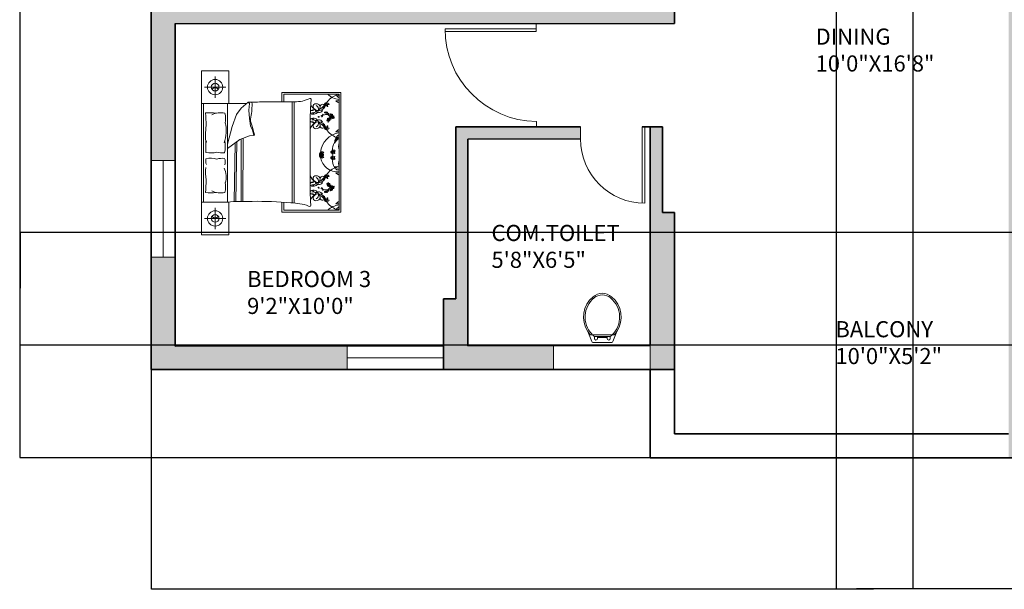
# Model space of a CAD drawing. Units: inches. Extents: x -26 to 13070, y -956 to 6917.
# Tile 1 of 13: x -26 to 341, y -956 to -744. Entities that reach past the tile are written whole.
import ezdxf

# ---------------------------------------------------------------- set-up
doc = ezdxf.new("R2010")
doc.units = ezdxf.units.IN
doc.header["$MEASUREMENT"] = 0
for name, color, linetype, lineweight in [('A-ANNO-DIMS', 2, 'Continuous', 18), ('A-AREA-IDEN', 7, 'Continuous', 18), ('A-DOOR', 3, 'Continuous', 18), ('A-FLOR-FIXT', 9, 'Continuous', 18), ('A-FURN', 8, 'Continuous', 13), ('A-GLAZ', 4, 'Continuous', 18), ('A-WALL', 7, 'Continuous', 35), ('A-WALL-PATT', 252, 'Continuous', 13)]:
    doc.layers.add(name, color=color, linetype=linetype, lineweight=lineweight)
doc.styles.get("Standard").update_dxf_attribs({"font": 'arial.ttf'})
doc.dimstyles.get("Standard").update_dxf_attribs({"dimtxt": 0.18, "dimasz": 0.18, "dimexe": 0.18, "dimexo": 0.0625, "dimgap": 0.09, "dimtad": 0, "dimtih": 1, "dimtoh": 1, "dimdec": 0, "dimzin": 0, "dimdsep": 46, "dimlunit": 3, "dimtxsty": 'Standard', "dimcen": 0.09, "dimadec": 0, "dimazin": 0, "dimtfac": 1, "dimtdec": 0, "dimtofl": 0, "dimtmove": 0, "dimatfit": 3, "dimfxl": 1, "dimtolj": 1, "dimtzin": 0, "dimarcsym": 0})

# ---------------------------------------------------------------- blocks, each defined once
blk = doc.blocks.new('WC-STANDARD')
for p, q in [((2.62, 2.77), (3.39, 2.77)), ((3.39, 2.77), (6.99, 2.77)), ((10.59, 2.77), (6.99, 2.77)), ((10.59, 2.77), (11.36, 2.77))]:
    blk.add_line(p, q)
for points in [[(1.63, 4.03, -0.383919), (3.55, 16.99, -0.163732), (6.99, 18.31, -0.359733)], [(3.02, 3.15, -0.431639), (3.9, 16.57, -0.162618), (6.99, 17.76, -0.470877)], [(12.35, 4.03, 0.383919), (10.43, 16.99, 0.163732), (6.99, 18.31, 0.359733)], [(10.59, 2.77, 0.448546), (10.08, 16.57, 0.162618), (6.99, 17.76, 0.470877)], [(2.62, 2.77, -0.040937), (1.63, 4.03, -0.163732)], [(6.99, 0), (3.49, 0, -0.31031), (3.07, 0.29), (1.63, 4.03, -0.209071)], [(6.99, 0), (10.49, 0, 0.31031), (10.92, 0.29), (12.35, 4.03, 0.209071)], [(11.36, 2.77, 0.040937), (12.35, 4.03, 0.163732)], [(3.39, 2.77, -0.014165), (3.02, 3.15, -0.162618)], [(4.02, 2.22, -0.022712), (3.39, 2.77, -0.162618)], [(6.99, 2.22), (4.02, 2.22, -0.022712)], [(4.02, 2.22), (4.02, 1.45, 1), (5.19, 1.45), (5.19, 1.85)], [(6.99, 2.22), (9.96, 2.22, 0.476108)], [(9.96, 2.22), (9.96, 1.45, -1), (8.79, 1.45), (8.79, 1.85)], [(9.96, 2.22, 0.022712), (10.59, 2.77, 0.162618)]]:
    blk.add_lwpolyline(points, format="xyb")
for points in [[(5.19, 1.85), (5.19, 2.22)], [(8.79, 1.85), (5.19, 1.85)], [(8.79, 1.85), (8.79, 2.22)]]:
    blk.add_lwpolyline(points)
blk = doc.blocks.new('WIN-36')
for p, q in [((0, 36), (0, 0)), ((9, 36), (0, 36)), ((4.5, 36), (4.5, 0)), ((9, 0), (9, 36)), ((0, 0), (9, 0))]:
    blk.add_line(p, q)
blk = doc.blocks.new('*D40')
at = {"layer": 'A-ANNO-DIMS', "color": 0, "lineweight": -2, "transparency": 16777216}
for p, q in [((22.64, -874.6), (22.64, -956.47)), ((547.64, -874.6), (547.64, -956.47)), ((22.82, -956.29), (284.85, -956.29)), ((547.46, -956.29), (285.43, -956.29))]:
    blk.add_line(p, q, dxfattribs=at)
at = {"layer": 'A-ANNO-DIMS', "color": 0, "transparency": 16777216}
for points in [[(22.82, -956.26), (22.82, -956.32), (22.64, -956.29)], [(547.46, -956.26), (547.46, -956.32), (547.64, -956.29)]]:
    blk.add_solid(points, dxfattribs=at)
at = {"layer": 'Defpoints', "color": 0, "transparency": 16777216}
for p in [(22.64, -874.54), (547.64, -874.54), (547.64, -956.29)]:
    blk.add_point(p, dxfattribs=at)
at = {"layer": 'A-ANNO-DIMS', "color": 0, "transparency": 16777216, "insert": (285.14, -956.29), "char_height": 0.18, "attachment_point": 5}
blk.add_mtext('\\A1;525', dxfattribs=at)
blk = doc.blocks.new('*D41')
at = {"layer": 'A-ANNO-DIMS', "color": 0, "lineweight": -2, "transparency": 16777216}
for p, q in [((214.58, 67.46), (-26.29, 67.46)), ((-26.11, 67.28), (-26.11, -419.86)), ((-26.11, -907.36), (-26.11, -420.22)), ((208.58, -907.54), (-26.29, -907.54))]:
    blk.add_line(p, q, dxfattribs=at)
at = {"layer": 'A-ANNO-DIMS', "color": 0, "transparency": 16777216}
for points in [[(-26.14, 67.28), (-26.08, 67.28), (-26.11, 67.46)], [(-26.14, -907.36), (-26.08, -907.36), (-26.11, -907.54)]]:
    blk.add_solid(points, dxfattribs=at)
at = {"layer": 'Defpoints', "color": 0, "transparency": 16777216}
for p in [(-26.11, 67.46), (214.64, 67.46), (208.64, -907.54)]:
    blk.add_point(p, dxfattribs=at)
at = {"layer": 'A-ANNO-DIMS', "color": 0, "transparency": 16777216, "insert": (-26.11, -420.04), "char_height": 0.18, "attachment_point": 5}
blk.add_mtext('\\A1;975', dxfattribs=at)
blk = doc.blocks.new('*D51')
at = {"layer": 'A-ANNO-DIMS', "color": 0, "lineweight": -2, "transparency": 16777216}
for p, q in [((277.92, -535.87), (277.92, -956.47)), ((306.46, -535.87), (306.46, -956.47)), ((278.1, -956.29), (291.8, -956.29)), ((306.28, -956.29), (292.59, -956.29))]:
    blk.add_line(p, q, dxfattribs=at)
at = {"layer": 'A-ANNO-DIMS', "color": 0, "transparency": 16777216}
for points in [[(278.1, -956.26), (278.1, -956.32), (277.92, -956.29)], [(306.28, -956.26), (306.28, -956.32), (306.46, -956.29)]]:
    blk.add_solid(points, dxfattribs=at)
at = {"layer": 'Defpoints', "color": 0, "transparency": 16777216}
for p in [(277.92, -535.8), (306.46, -535.8), (306.46, -956.29)]:
    blk.add_point(p, dxfattribs=at)
at = {"layer": 'A-ANNO-DIMS', "color": 0, "transparency": 16777216, "insert": (292.19, -956.29), "char_height": 0.18, "attachment_point": 5}
blk.add_mtext('\\A1;28.54', dxfattribs=at)
blk = doc.blocks.new('*D59')
at = {"layer": 'A-ANNO-DIMS', "color": 0, "lineweight": -2, "transparency": 16777216}
for p, q in [((538.58, -823.54), (-26.29, -823.54)), ((-26.11, -823.72), (-26.11, -844.36)), ((-26.11, -865.36), (-26.11, -844.72)), ((538.58, -865.54), (-26.29, -865.54))]:
    blk.add_line(p, q, dxfattribs=at)
at = {"layer": 'A-ANNO-DIMS', "color": 0, "transparency": 16777216}
for points in [[(-26.14, -823.72), (-26.08, -823.72), (-26.11, -823.54)], [(-26.14, -865.36), (-26.08, -865.36), (-26.11, -865.54)]]:
    blk.add_solid(points, dxfattribs=at)
at = {"layer": 'Defpoints', "color": 0, "transparency": 16777216}
for p in [(-26.11, -823.54), (538.64, -823.54), (538.64, -865.54)]:
    blk.add_point(p, dxfattribs=at)
at = {"layer": 'A-ANNO-DIMS', "color": 0, "transparency": 16777216, "insert": (-26.11, -844.54), "char_height": 0.18, "attachment_point": 5}
blk.add_mtext('\\A1;42', dxfattribs=at)

msp = doc.modelspace()

# ---------------------------------------------------------------- hatches: boundary and pattern name
at = {"layer": 'A-WALL-PATT'}
h = msp.add_hatch(color=256, dxfattribs=at)
h.dxf.hatch_style = 1
h.paths.add_polyline_path([(223.641, 10.458), (214.641, 10.458), (22.641, 10.458), (22.641, -171.042), (31.641, -171.042), (31.641, -135.042), (205.641, -135.042), (205.641, -241.042), (210.141, -241.042), (210.141, -130.542), (94.641, -130.542), (94.641, -76.542), (85.641, -76.542), (85.641, -126.042), (27.141, -126.042), (27.141, 5.958), (85.641, 5.958), (85.641, -52.542), (94.641, -52.542), (94.641, 1.458), (214.641, 1.458), (214.641, -16.542), (223.641, -16.542), (229.641, -16.542), (229.641, -7.542), (223.641, -7.542)])
h.paths.add_polyline_path([(367.048, 10.458), (346.641, 10.458), (337.641, 10.458), (337.641, -7.542), (331.641, -7.542), (331.641, -16.542), (337.641, -16.542), (342.141, -16.542), (342.141, -128.542), (346.641, -128.542), (346.641, 1.458), (367.048, 1.458)])
h.paths.add_polyline_path([(547.641, 10.458), (403.048, 10.458), (403.048, 1.458), (538.641, 1.458), (538.641, -46.542), (547.641, -46.542)])
h.paths.add_polyline_path([(547.641, -106.542), (538.641, -106.542), (538.641, -154.542), (481.013, -154.542), (481.013, -159.042), (538.641, -159.042), (547.641, -159.042)])
h.paths.add_polyline_path([(457.013, -154.542), (342.141, -154.542), (342.141, -165.042), (346.641, -165.042), (346.641, -159.042), (414.141, -159.042), (414.141, -225.042), (346.641, -225.042), (346.641, -189.042), (342.141, -189.042), (342.141, -234.042), (390.641, -234.042), (390.641, -286.042), (395.141, -286.042), (395.141, -234.042), (456.141, -234.042), (456.141, -312.042), (372.641, -312.042), (372.641, -316.542), (462.641, -316.542), (462.641, -312.042), (460.641, -312.042), (460.641, -234.042), (538.641, -234.042), (547.641, -234.042), (547.641, -195.042), (538.641, -195.042), (538.641, -225.042), (418.641, -225.042), (418.641, -159.042), (457.013, -159.042)])
h.paths.add_polyline_path([(547.641, -270.042), (538.641, -270.042), (538.641, -312.042), (486.641, -312.042), (486.641, -316.542), (538.641, -316.542), (547.641, -316.542)], flags=0)
h.paths.add_polyline_path([(547.641, -456.306), (538.641, -456.306), (538.641, -457.542), (346.641, -457.542), (346.641, -316.542), (346.641, -312.042), (342.141, -312.042), (342.141, -457.542), (145.641, -457.542), (145.641, -466.542), (342.141, -466.542), (342.141, -627.042), (346.641, -627.042), (346.641, -466.542), (538.641, -466.542), (538.641, -514.542), (547.641, -514.542)])
h.paths.add_polyline_path([(466.641, -622.542), (372.641, -622.542), (372.641, -627.042), (388.641, -627.042), (388.641, -721.542), (393.141, -721.542), (393.141, -627.042), (462.141, -627.042), (462.141, -717.042), (466.641, -717.042)])
h.paths.add_polyline_path([(547.641, -574.542), (538.641, -574.542), (538.641, -622.542), (492.641, -622.542), (492.641, -627.042), (538.641, -627.042), (538.641, -654.042), (547.641, -654.042)])
h.paths.add_polyline_path([(547.641, -690.042), (538.641, -690.042), (538.641, -717.042), (466.641, -717.042), (466.641, -721.542), (538.641, -721.542), (538.641, -763.542), (547.641, -763.542)])
h.paths.add_polyline_path([(462.141, -717.042), (419.141, -717.042), (419.141, -721.542), (462.141, -721.542)], flags=0)
h.paths.add_polyline_path([(346.641, -721.542), (352.641, -721.542), (352.641, -717.042), (342.141, -717.042), (342.141, -874.542), (342.141, -907.542), (351.141, -907.542), (351.141, -874.542), (395.949, -874.542), (395.949, -865.542), (351.141, -865.542), (351.141, -841.542), (346.641, -841.542)])
h.paths.add_polyline_path([(547.641, -823.542), (538.641, -823.542), (538.641, -865.542), (431.949, -865.542), (431.949, -874.542), (547.641, -874.542)])
h.paths.add_polyline_path([(172.641, -865.713), (140.641, -865.744), (140.641, -788.744), (182.646, -788.704), (182.641, -784.204), (136.141, -784.249), (136.141, -848.332), (131.641, -848.332), (131.641, -874.542), (172.641, -874.542)])
h.paths.add_polyline_path([(217.641, -816.13), (213.141, -816.13), (213.141, -784.174), (208.641, -784.179), (208.641, -865.679), (208.641, -874.542), (217.641, -874.542)])
h.paths.add_polyline_path([(95.641, -865.788), (31.641, -865.849), (31.641, -832.695), (22.641, -832.695), (22.641, -874.542), (95.641, -874.542)])
h.paths.add_polyline_path([(217.641, -741.17), (31.641, -741.349), (31.641, -708.349), (22.641, -708.349), (22.641, -772.542), (22.641, -796.695), (31.641, -796.695), (31.641, -763.542), (31.641, -745.849), (217.641, -745.67)])
h.paths.add_polyline_path([(31.641, -651.349), (99.65, -651.284), (99.641, -642.284), (31.641, -642.349), (31.641, -639.042), (31.641, -588.349), (125.641, -588.259), (125.641, -651.259), (134.641, -651.25), (134.641, -579.25), (112.641, -579.271), (112.641, -549.042), (112.641, -504.271), (85.633, -504.297), (85.641, -513.297), (103.641, -513.28), (103.641, -549.042), (103.641, -579.28), (31.641, -579.349), (31.641, -549.042), (31.641, -513.349), (49.641, -513.314), (49.633, -504.332), (31.641, -504.349), (22.641, -504.358), (22.641, -684.349), (31.641, -684.349)])
h.paths.add_polyline_path([(31.641, -276.042), (145.641, -276.042), (145.641, -402.042), (145.641, -419.542), (154.641, -419.542), (154.641, -411.042), (154.641, -271.542), (210.141, -271.542), (210.141, -265.042), (205.641, -265.042), (205.641, -267.042), (31.641, -267.042), (31.641, -231.042), (22.641, -231.042), (22.641, -426.852), (31.641, -426.852), (31.641, -411.042), (31.641, -402.042)])

# ---------------------------------------------------------------- linework, layer by layer
at = {"layer": 'A-DOOR'}
for p, q in [((166.16, -747.72), (132.16, -747.72)), ((166.16, -745.72), (166.16, -748.72)), ((166.16, -748.72), (132.16, -748.72)), ((166.197, -784.22), (166.197, -782.22)), ((182.641, -784.179), (182.646, -788.704)), ((205.641, -788.679), (205.641, -784.179)), ((206.641, -788.679), (206.641, -784.179)), ((205.641, -788.679), (205.641, -812.679)), ((206.641, -788.679), (206.641, -812.679))]:
    msp.add_line(p, q, dxfattribs=at)
for centre, radius, start, end in [((166.664, -747.72), 34.503, 180, 269.22602), ((206.641, -788.683), 23.996, 180.04936, 270)]:
    msp.add_arc(centre, radius, start, end, dxfattribs=at)
at = {"layer": 'A-FURN'}
for p, q in [((41.423, -763.315), (41.423, -824.436)), ((46.517, -773.421), (46.517, -765.434)), ((50.51, -769.427), (42.524, -769.427)), ((71.385, -771.383), (71.385, -774.84)), ((93.403, -771.383), (71.385, -771.383)), ((72.093, -774.839), (72.093, -772.091)), ((72.093, -772.091), (92.695, -772.091)), ((92.695, -772.091), (92.695, -815.234)), ((93.403, -815.942), (93.403, -771.383)), ((41.423, -775.539), (58.199, -775.539)), ((42.208, -812.212), (42.208, -775.539)), ((51.082, -775.539), (51.082, -812.212)), ((56.239, -777.221), (54.507, -779.573)), ((58.837, -774.992), (56.239, -777.221)), ((59.332, -775.487), (58.837, -774.992)), ((59.085, -777.963), (59.332, -775.487)), ((75.197, -812.49), (75.197, -774.835)), ((75.96, -812.548), (75.96, -774.835)), ((54.507, -779.573), (52.899, -784.029)), ((59.332, -781.058), (59.085, -777.963)), ((59.703, -783.782), (59.332, -781.058)), ((86.498, -778.114), (85.807, -777.979)), ((52.899, -784.029), (51.082, -790.694)), ((60.446, -785.391), (59.703, -783.782)), ((81.963, -806.284), (81.963, -781.468)), ((86.498, -782.386), (85.807, -782.521)), ((55.744, -788.981), (59.332, -787.62)), ((56.801, -811.996), (56.897, -788.544)), ((59.332, -787.62), (60.941, -787.372)), ((60.941, -787.372), (60.446, -785.391)), ((51.082, -792.331), (55.744, -788.981)), ((53.622, -812.048), (53.927, -790.287)), ((54.249, -812.024), (54.562, -789.831)), ((56.173, -811.993), (56.265, -788.784)), ((86.498, -804.939), (85.807, -804.804)), ((86.498, -809.211), (85.807, -809.346)), ((46.517, -814.331), (46.517, -822.317)), ((71.385, -812.553), (71.385, -815.942)), ((72.093, -815.234), (72.093, -812.54)), ((71.385, -815.942), (93.403, -815.942)), ((92.695, -815.234), (72.093, -815.234)), ((50.51, -818.324), (42.524, -818.324))]:
    msp.add_line(p, q, dxfattribs=at)
for points in [[(51.61, -775.539), (51.61, -763.315), (41.423, -763.315)], [(46.517, -769.427), (45.282, -770.14)], [(46.517, -769.427), (47.752, -770.14)], [(41.423, -812.212), (51.61, -812.212), (51.61, -824.436), (41.423, -824.436)], [(46.517, -818.324), (45.282, -817.611)], [(46.517, -818.324), (47.752, -817.611)]]:
    msp.add_lwpolyline(points, dxfattribs=at)
for points in [[(64.434, -774.864, -0.0012423), (76.031, -774.835, 0.1272016), (81.811, -773.61)], [(42.947, -779.05, -0.0748968), (46.939, -779.124, 0.4728166)], [(47.162, -793.589, -0.1409896), (43.09, -793.712, -0.2352448)], [(47.162, -796.2, 0.1409896), (43.09, -796.077, 0.2352448)], [(42.947, -808.702, 0.0748968), (46.939, -808.627, -0.4728166)], [(74.716, -812.473, -0.0561118), (78.079, -812.916, -0.0953413), (81.318, -813.776)]]:
    msp.add_lwpolyline(points, format="xyb", dxfattribs=at)
for centre, radius in [((46.517, -769.427), 2.852), ((46.517, -769.427), 1.426), ((90.353, -780.627), 0.156), ((88.713, -781.645), 0.156), ((88.713, -805.68), 0.156), ((90.353, -806.698), 0.156), ((46.517, -818.324), 2.852), ((46.517, -818.324), 1.426)]:
    msp.add_circle(centre, radius, dxfattribs=at)
for centre, radius, start, end in [((81.772, -774.172), 0.564, 332.65876, 86.02002), ((94.559, -779.804), 7.982, 111.40921, 145.61345), ((93.77, -766.149), 7.982, 228.1144, 262.25504), ((94.839, -770.153), 3.889, 209.88843, 236.53828), ((95.564, -768.754), 4.847, 223.51858, 233.69643), ((60.357, -718.951), 56.062, 268.44695, 274.17059), ((37.193, -776.038), 23.068, 348.6608, 2.54812), ((145.587, -780.738), 63.628, 174.31131, 180.65675), ((86.268, -773.934), 4.626, 206.70034, 236.33288), ((84.046, -776.629), 1.032, 88.94622, 185.51443), ((84.81, -776.312), 1.838, 193.079, 274.70666), ((84.194, -777.052), 1.461, 7.11425, 95.05515), ((83.64, -777.626), 1.418, 338.57785, 68.41813), ((83.869, -776.798), 1.775, 305.95986, 357.6409), ((84.761, -774.87), 3.28, 273.4924, 303.71172), ((84.528, -774.897), 2.886, 288.2955, 328.73863), ((86.548, -776.716), 0.917, 19.13116, 189.73602), ((86.271, -776.496), 1.145, 285.6955, 4.03098), ((87.794, -777.73), 1.22, 128.41745, 173.8338), ((87.541, -776.527), 0.562, 126.73195, 206.02445), ((87.816, -775.939), 0.662, 76.27204, 177.04841), ((86.809, -774.586), 1.363, 284.70312, 328.61733), ((88.71, -776.32), 1.262, 125.76571, 194.53465), ((82.522, -774.086), 5.584, 332.81761, 347.48274), ((88.161, -776.161), 0.885, 20.96132, 102.28847), ((88.639, -775.276), 0.667, 181.71311, 301.53669), ((86.453, -776.625), 2.019, 2.0648, 41.15983), ((87.669, -775.874), 0.653, 316.22381, 62.3173), ((88.078, -776.266), 0.0863, 20.28165, 316.22381), ((88.371, -776.556), 0.0991, 168.5166, 2.0648), ((88.321, -776.545), 0.0482, 52.05911, 168.5166), ((93.939, -772.331), 3.245, 221.04544, 247.44526), ((92.195, -763.442), 11.043, 266.34809, 272.59189), ((-538.724, -812.74), 582.646, 2.850225, 3.314791), ((48.542, -786.837), 7.878, 78.24166, 114.8684), ((42.231, -781.23), 8.191, 348.96311, 14.89607), ((64.689, -781.552), 4.975, 168.6608, 203.73842), ((82.64, -781.733), 0.736, 134.45169, 156.77099), ((82.64, -778.767), 0.736, 206.44199, 225.54831), ((82.64, -778.767), 0.736, 127.67503, 149.9707), ((82.416, -775.631), 2.532, 260.84458, 301.17822), ((83.074, -777.592), 1.948, 240.8249, 340.71782), ((82.494, -778.456), 0.915, 246.16459, 318.43469), ((83.074, -782.908), 1.948, 19.28218, 119.1751), ((82.494, -782.044), 0.915, 41.56531, 113.83541), ((83.515, -780.134), 2.357, 85.26963, 124.21495), ((83.426, -777.298), 1.757, 240.08513, 262.56401), ((84.115, -779.894), 1.253, 74.85287, 138.43469), ((85.181, -777.356), 1.52, 196.8663, 330.09146), ((84.542, -778.319), 0.379, 254.85287, 12.69594), ((83.515, -780.134), 2.357, 53.65552, 57.29887), ((85.045, -780.412), 0.192, 169.58644, 349.56155), ((85.117, -780.425), 0.118, 349.56155, 167.29493), ((88.194, -784.662), 5.062, 110.10592, 116.9968), ((86.496, -780.489), 0.321, 129.50559, 182.64212), ((85.575, -779.747), 0.966, 308.43876, 328.83597), ((85.406, -778.962), 1.724, 296.50636, 305.31021), ((85.392, -779.848), 0.982, 336.39009, 344.48709), ((86.462, -780.099), 0.125, 83.94573, 185.62162), ((85.963, -779.982), 0.512, 328.83597, 0.81412), ((86.228, -780.132), 0.293, 306.52319, 32.46683), ((86.578, -779.905), 0.125, 112.55835, 214.23425), ((86.497, -779.682), 0.293, 265.71315, 351.65678), ((86.24, -779.52), 0.512, 297.36586, 329.34401), ((85.852, -779.08), 0.982, 313.69288, 321.78988), ((86.938, -779.75), 0.321, 115.53786, 168.67439), ((85.849, -779.289), 0.966, 329.34401, 349.74122), ((88.194, -784.662), 5.062, 86.17232, 106.41582), ((85.077, -779.511), 1.724, 352.86976, 1.67361), ((87.361, -778.889), 0.12, 125.0752, 284.76444), ((87.547, -778.843), 0.26, 127.3642, 168.43627), ((87.343, -778.634), 0.374, 277.49685, 341.27373), ((87.64, -778.809), 0.149, 88.13253, 178.89195), ((87.939, -778.967), 0.322, 136.34618, 189.6513), ((87.754, -778.998), 0.134, 189.6513, 312.32085), ((87.788, -778.628), 0.156, 183.27684, 356.72316), ((88.274, -778.906), 0.51, 164.28291, 186.91484), ((87.673, -778.909), 0.255, 312.32085, 40.21108), ((88.213, -778.622), 0.362, 201.63824, 274.94696), ((87.734, -779.117), 0.473, 42.38963, 66.57243), ((92.501, -775.377), 5.803, 217.9541, 226.84587), ((88.076, -778.84), 0.257, 10.95974, 52.23791), ((88.233, -778.864), 0.119, 274.94696, 37.52629), ((88.481, -780.454), 0.71, 253.63009, 325.46314), ((88.681, -781.439), 0.502, 82.07481, 142.68955), ((88.624, -780.749), 0.516, 228.34199, 274.98936), ((88.439, -781.45), 0.153, 138.29465, 276.24744), ((88.496, -781.473), 0.212, 358.57189, 143.89544), ((88.62, -781.306), 0.214, 208.84925, 269.93549), ((88.635, -779.541), 0.125, 112.55835, 214.23425), ((88.554, -779.318), 0.293, 265.71315, 351.65678), ((88.296, -779.156), 0.512, 297.36586, 329.34401), ((88.321, -782.14), 2.538, 60.79592, 85.24398), ((82.918, -785.794), 8.351, 37.82556, 47.75876), ((87.909, -778.716), 0.982, 313.69288, 321.78988), ((88.64, -780.832), 0.431, 273.87739, 357.15012), ((88.995, -779.386), 0.321, 115.53786, 168.67439), ((89.183, -781.604), 0.491, 121.9501, 165.24419), ((87.906, -778.925), 0.966, 329.34401, 349.74122), ((88.807, -780.528), 0.418, 262.07481, 308.23927), ((88.844, -781.415), 0.103, 262.86802, 7.09399), ((87.134, -779.147), 1.724, 352.86976, 1.67361), ((88.831, -781.328), 0.307, 278.56141, 22.59143), ((91.692, -782.401), 3.044, 156.15226, 156.94993), ((89.005, -781.318), 0.154, 44.37319, 121.9501), ((89.481, -780.956), 0.431, 181.4625, 249.4747), ((89.407, -780.616), 0.418, 215.11283, 261.27729), ((89.741, -780.638), 0.71, 197.88895, 269.722), ((91.692, -782.401), 3.044, 130.18202, 149.45598), ((89.52, -780.88), 0.516, 248.36273, 295.0101), ((89.268, -781.525), 0.502, 20.66254, 81.27729), ((89.558, -779.494), 0.174, 33.09787, 123.13641), ((85.729, -781.945), 4.547, 31.11559, 34.8118), ((89.306, -779.793), 0.471, 2.31716, 70.52013), ((90.016, -780.667), 0.502, 139.38119, 199.99593), ((89.08, -780.303), 0.71, 310.93647, 22.76952), ((89.405, -780.342), 0.516, 285.64837, 332.29574), ((89.694, -779.908), 0.136, 135.73542, 318.12966), ((89.468, -779.688), 0.18, 315.73542, 31.11559), ((89.318, -780.069), 0.418, 319.38119, 5.54564), ((89.796, -779.908), 0.136, 68.24522, 250.63946), ((89.484, -779.74), 0.405, 352.60083, 57.18452), ((90.931, -782.46), 2.711, 111.70871, 116.21806), ((88.321, -782.14), 2.538, 47.50829, 55.99666), ((89.871, -779.649), 0.405, 252.8042, 349.69432), ((89.484, -780.374), 0.431, 331.18377, 51.67918), ((89.927, -780.889), 0.12, 125.0752, 284.76444), ((89.913, -779.615), 0.18, 248.24522, 323.62539), ((90.112, -780.842), 0.26, 93.63497, 168.43627), ((90.079, -780.432), 0.153, 138.29465, 276.24744), ((89.755, -779.504), 0.471, 291.70871, 3.02993), ((89.909, -780.634), 0.374, 277.49685, 341.27373), ((90.137, -780.455), 0.212, 358.57189, 143.89544), ((90.206, -780.808), 0.149, 88.13253, 178.89195), ((86.397, -777.024), 4.547, 323.62539, 327.3216), ((90.26, -780.288), 0.214, 208.84925, 269.93549), ((90.078, -780.339), 0.245, 274.21229, 318.15875), ((90.505, -780.966), 0.322, 136.34618, 189.6513), ((90.32, -780.998), 0.134, 189.6513, 312.32085), ((90.126, -779.623), 0.174, 325.60767, 55.6462), ((90.84, -780.905), 0.51, 164.28291, 186.91484), ((90.824, -780.586), 0.491, 121.9501, 165.24419), ((90.239, -780.909), 0.255, 312.32085, 40.21108), ((90.778, -780.622), 0.362, 201.63824, 274.94696), ((90.485, -780.397), 0.103, 262.86802, 7.09399), ((90.299, -781.117), 0.473, 42.38963, 66.57243), ((90.472, -780.31), 0.307, 278.56141, 22.59143), ((90.642, -780.839), 0.257, 10.95974, 118.78041), ((90.646, -780.3), 0.154, 44.37319, 121.9501), ((90.799, -780.863), 0.119, 274.94696, 37.52629), ((65.064, -787.425), 22.167, 170.50302, 187.78042), ((36.409, -785.542), 14.207, 340.73848, 11.96026), ((37.844, -791.616), 23.703, 10.66171, 19.88058), ((82.64, -781.733), 0.736, 203.28564, 232.32497), ((82.416, -784.869), 2.532, 58.82178, 100.28665), ((86.268, -786.566), 4.626, 123.66712, 158.50587), ((83.515, -780.366), 2.357, 235.78505, 274.73037), ((83.426, -783.202), 1.757, 97.43599, 119.91487), ((84.046, -783.871), 1.032, 174.48557, 271.05378), ((84.81, -784.188), 1.838, 85.29334, 166.921), ((84.115, -780.606), 1.253, 221.56531, 285.14713), ((85.181, -783.143), 1.52, 29.90854, 163.1337), ((84.194, -783.448), 1.461, 264.94485, 352.88575), ((83.64, -782.874), 1.418, 291.58187, 21.42215), ((84.542, -782.181), 0.379, 347.30406, 105.14713), ((83.515, -780.366), 2.357, 302.70113, 306.34448), ((83.869, -783.702), 1.775, 2.3591, 54.04014), ((84.761, -785.629), 3.28, 56.28828, 86.5076), ((84.528, -785.602), 2.886, 31.26137, 71.7045), ((86.548, -783.784), 0.917, 170.26398, 340.86884), ((87.794, -782.77), 1.22, 186.1662, 231.58255), ((86.271, -784.004), 1.145, 355.96902, 74.3045), ((87.541, -783.973), 0.562, 153.97555, 233.26805), ((87.816, -784.561), 0.662, 182.95159, 283.72796), ((86.809, -785.913), 1.363, 31.38267, 75.29688), ((88.71, -784.18), 1.262, 165.46535, 234.23429), ((82.522, -786.414), 5.584, 12.51726, 27.18239), ((86.453, -783.875), 2.019, 318.84017, 357.9352), ((87.669, -784.625), 0.653, 297.6827, 43.77619), ((88.639, -785.223), 0.667, 58.46331, 178.28689), ((88.161, -784.339), 0.885, 257.71153, 339.03868), ((88.045, -784.243), 0.052, 43.77292, 339.73329), ((88.286, -781.907), 0.12, 125.0752, 284.76444), ((88.472, -781.86), 0.26, 93.63497, 168.43627), ((88.371, -783.944), 0.0991, 357.9352, 191.4834), ((88.321, -783.954), 0.0482, 191.4834, 307.94089), ((88.268, -781.652), 0.374, 277.49685, 341.27373), ((88.565, -781.827), 0.149, 88.13253, 178.89195), ((88.437, -781.357), 0.245, 274.21229, 318.15875), ((88.864, -781.985), 0.322, 136.34618, 189.6513), ((88.679, -782.016), 0.134, 189.6513, 312.32085), ((91.692, -782.401), 3.044, 175.24147, 182.89291), ((89.199, -781.923), 0.51, 164.28291, 186.91484), ((88.598, -781.927), 0.255, 312.32085, 40.21108), ((89.138, -781.64), 0.362, 201.63824, 274.94696), ((88.659, -782.135), 0.473, 42.38963, 66.57243), ((89.001, -781.857), 0.257, 10.95974, 118.78041), ((89.158, -781.881), 0.119, 274.94696, 37.52629), ((60.991, -787.233), 0.147, 250.24637, 1.13765), ((93.77, -794.351), 7.982, 97.74496, 175.53767), ((94.559, -780.696), 7.982, 214.38655, 248.59079), ((94.839, -790.347), 3.889, 123.46172, 178.72803), ((95.564, -791.746), 4.847, 126.30357, 162.14962), ((96.927, -794.293), 7.209, 125.94696, 145.98766), ((93.939, -788.169), 3.245, 112.55474, 138.95456), ((92.195, -797.058), 11.043, 87.40811, 93.65191), ((53.862, -792.107), 10.891, 166.04004, 188.47507), ((39.511, -791.294), 10.778, 346.37624, 10.13831), ((98.045, -793.74), 7.982, 152.5854, 175.53767), ((96.891, -791.508), 4.389, 162.9798, 196.45689), ((45.995, -796.916), 3.024, 163.89744, 206.65626), ((49.205, -786.384), 7.489, 254.17072, 275.98711), ((49.205, -803.405), 7.489, 84.01289, 105.82928), ((47.049, -797.325), 3.24, 341.45927, 24.98174), ((85.997, -794.365), 0.662, 106.19625, 206.97263), ((85.997, -794.997), 0.662, 153.02737, 253.80375), ((84.45, -793.695), 1.363, 314.62734, 358.54154), ((84.45, -795.667), 1.363, 1.45846, 45.37266), ((86.963, -794.249), 1.262, 155.68992, 224.45887), ((86.963, -795.113), 1.262, 135.54113, 204.31008), ((86.407, -794.386), 0.885, 50.88554, 132.21268), ((86.38, -793.38), 0.667, 211.63732, 331.4609), ((85.838, -794.382), 0.653, 346.14802, 92.24151), ((80.485, -795.4), 5.584, 2.74183, 17.40696), ((85.158, -795.64), 2.019, 31.98902, 71.08405), ((80.485, -793.962), 5.584, 342.59304, 357.25817), ((85.158, -793.723), 2.019, 288.91595, 328.01098), ((85.838, -794.98), 0.653, 267.75849, 13.85198), ((86.38, -795.982), 0.667, 28.5391, 148.36268), ((86.407, -794.977), 0.885, 227.78732, 309.11446), ((91.927, -794.754), 6.177, 188.18034, 277.13645), ((86.388, -794.518), 0.0863, 50.07546, 346.14802), ((86.355, -794.836), 0.052, 13.97912, 309.80908), ((86.738, -794.639), 0.0482, 81.98332, 198.44082), ((86.738, -794.724), 0.0482, 161.55918, 278.01668), ((86.786, -794.623), 0.0991, 198.44082, 31.98902), ((86.786, -794.74), 0.0991, 328.01098, 161.55918), ((90.272, -793.754), 0.662, 106.19625, 206.97263), ((90.272, -795.608), 0.662, 153.02737, 253.80375), ((88.725, -793.084), 1.363, 314.62734, 358.54154), ((88.725, -796.278), 1.363, 1.45846, 45.37266), ((91.238, -793.638), 1.262, 155.68992, 224.45887), ((91.238, -795.724), 1.262, 135.54113, 204.31008), ((90.683, -793.774), 0.885, 50.88554, 132.21268), ((90.655, -792.769), 0.667, 211.63732, 331.4609), ((90.113, -793.771), 0.653, 346.14802, 92.24151), ((89.433, -795.028), 2.019, 31.98902, 71.08405), ((84.76, -794.789), 5.584, 2.74183, 17.40696), ((84.76, -794.573), 5.584, 342.59304, 357.25817), ((89.433, -794.334), 2.019, 288.91595, 328.01098), ((90.113, -795.591), 0.653, 267.75849, 13.85198), ((90.655, -796.593), 0.667, 28.5391, 148.36268), ((90.663, -793.907), 0.0863, 50.07546, 346.14802), ((90.63, -795.447), 0.052, 13.97912, 309.80908), ((91.013, -794.028), 0.0482, 81.98332, 198.44082), ((91.013, -795.335), 0.0482, 161.55918, 278.01668), ((91.061, -794.012), 0.0991, 198.44082, 31.98902), ((91.061, -795.351), 0.0991, 328.01098, 161.55918), ((99.153, -793.246), 6.49, 174.36426, 175.62128), ((103.599, -796.665), 11.598, 160.09716, 160.27829), ((53.642, -801.447), 10.745, 168.8159, 193.65729), ((42.835, -802.986), 7.78, 343.82536, 26.12389), ((94.559, -806.629), 7.982, 111.40921, 145.61345), ((90.683, -795.588), 0.885, 227.78732, 309.11446), ((98.045, -795.623), 7.982, 184.46233, 207.4146), ((91.363, -795.552), 3.573, 263.38046, 291.88297), ((92.357, -798.83), 1.433, 190.92615, 283.61018), ((92.161, -797.754), 1.812, 228.09513, 287.13912), ((96.891, -797.855), 4.389, 163.54311, 197.0202), ((99.153, -796.116), 6.49, 184.37872, 185.63574), ((103.599, -792.698), 11.598, 199.72171, 199.90284), ((86.268, -800.759), 4.626, 201.49413, 236.33288), ((84.046, -803.454), 1.032, 88.94622, 185.51443), ((84.194, -803.877), 1.461, 7.11425, 95.05515), ((83.64, -804.451), 1.418, 338.57785, 68.41813), ((84.528, -801.723), 2.886, 288.2955, 328.73863), ((86.548, -803.541), 0.917, 19.13116, 189.73602), ((86.271, -803.321), 1.145, 285.6955, 4.03098), ((87.541, -803.353), 0.562, 126.73195, 206.02445), ((87.816, -802.764), 0.662, 76.27204, 177.04841), ((86.809, -801.412), 1.363, 284.70312, 328.61733), ((88.71, -803.145), 1.262, 125.76571, 194.53465), ((82.522, -800.911), 5.584, 332.81761, 347.48274), ((88.161, -802.986), 0.885, 20.96132, 102.28847), ((87.669, -802.7), 0.653, 316.22381, 62.3173), ((86.453, -803.45), 2.019, 2.0648, 41.15983), ((88.639, -802.102), 0.667, 181.71311, 301.53669), ((88.078, -803.092), 0.0863, 20.28165, 316.22381), ((88.371, -803.381), 0.0991, 168.5166, 2.0648), ((88.321, -803.371), 0.0482, 52.05911, 168.5166), ((92.195, -790.267), 11.043, 266.34809, 272.59189), ((93.939, -799.156), 3.245, 221.04544, 247.44526), ((-538.724, -775.012), 582.646, 356.685209, 357.149775), ((42.231, -806.521), 8.191, 345.10393, 11.03689), ((141.409, -808.156), 59.476, 178.19649, 184.75976), ((82.416, -802.456), 2.532, 259.71335, 301.17822), ((82.64, -805.593), 0.736, 127.67503, 156.71436), ((82.64, -805.593), 0.736, 203.28564, 225.54831), ((83.074, -804.417), 1.948, 240.8249, 340.71782), ((82.494, -805.281), 0.915, 246.16459, 318.43469), ((83.515, -806.959), 2.357, 85.26963, 124.21495), ((83.426, -804.123), 1.757, 240.08513, 262.56401), ((84.81, -803.137), 1.838, 193.079, 274.70666), ((84.115, -806.72), 1.253, 74.85287, 138.43469), ((85.181, -804.182), 1.52, 196.8663, 330.09146), ((84.542, -805.144), 0.379, 254.85287, 12.69594), ((83.515, -806.959), 2.357, 53.65552, 57.29887), ((85.045, -806.913), 0.192, 10.43845, 190.41356), ((83.869, -803.623), 1.775, 305.95986, 357.6409), ((84.761, -801.696), 3.28, 273.4924, 303.71172), ((85.117, -806.9), 0.118, 192.70507, 10.43845), ((85.575, -807.578), 0.966, 31.16403, 51.56124), ((86.496, -806.836), 0.321, 177.35788, 230.49441), ((85.406, -808.363), 1.724, 54.68979, 63.49364), ((85.392, -807.477), 0.982, 15.51291, 23.60991), ((85.963, -807.343), 0.512, 359.18588, 31.16403), ((86.228, -807.193), 0.293, 327.53317, 53.47681), ((87.794, -804.555), 1.22, 128.41745, 173.8338), ((88.286, -805.418), 0.12, 75.23556, 234.9248), ((88.472, -805.465), 0.26, 191.56373, 266.36503), ((88.624, -806.576), 0.516, 85.01064, 131.65801), ((88.481, -806.871), 0.71, 34.53686, 106.36991), ((88.681, -805.886), 0.502, 217.31045, 277.92519), ((88.439, -805.875), 0.153, 83.75256, 221.70535), ((88.268, -805.673), 0.374, 18.72627, 82.50315), ((88.496, -805.852), 0.212, 216.10456, 1.42811), ((88.565, -805.498), 0.149, 181.10805, 271.86747), ((88.62, -806.019), 0.214, 90.06451, 151.15075), ((88.437, -805.968), 0.245, 41.84125, 85.78771), ((82.918, -801.532), 8.351, 312.24124, 322.17444), ((88.864, -805.341), 0.322, 170.3487, 223.65382), ((88.679, -805.309), 0.134, 47.67915, 170.3487), ((91.692, -804.924), 3.044, 177.10709, 184.75853), ((88.64, -806.493), 0.431, 2.84988, 86.12261), ((89.199, -805.402), 0.51, 173.08516, 195.71709), ((89.183, -805.721), 0.491, 194.75581, 238.0499), ((88.807, -806.797), 0.418, 51.76073, 97.92519), ((88.598, -805.398), 0.255, 319.78892, 47.67915), ((89.138, -805.685), 0.362, 85.05304, 158.36176), ((88.844, -805.91), 0.103, 352.90601, 97.13198), ((88.659, -805.19), 0.473, 293.42757, 317.61037), ((89.001, -805.468), 0.257, 241.21959, 349.04026), ((88.831, -805.997), 0.307, 337.40857, 81.43859), ((91.692, -804.924), 3.044, 203.05007, 203.84774), ((89.005, -806.007), 0.154, 238.0499, 315.62681), ((89.481, -806.37), 0.431, 110.5253, 178.5375), ((89.741, -806.687), 0.71, 90.278, 162.11105), ((89.407, -806.709), 0.418, 98.72271, 144.88717), ((91.692, -804.924), 3.044, 210.54402, 229.81798), ((89.158, -805.444), 0.119, 322.47371, 85.05304), ((89.52, -806.445), 0.516, 64.9899, 111.63727), ((89.268, -805.801), 0.502, 278.72271, 339.33746), ((90.016, -806.658), 0.502, 160.00407, 220.61881), ((89.08, -807.022), 0.71, 337.23048, 49.06353), ((89.405, -806.983), 0.516, 27.70426, 74.35163), ((89.318, -807.256), 0.418, 354.45436, 40.61881), ((88.321, -805.185), 2.538, 304.00334, 312.49171), ((89.484, -806.951), 0.431, 308.32082, 28.81623), ((89.927, -806.436), 0.12, 75.23556, 234.9248), ((90.112, -806.483), 0.26, 191.56373, 266.36503), ((90.079, -806.893), 0.153, 83.75256, 221.70535), ((89.909, -806.691), 0.374, 18.72627, 82.50315), ((90.137, -806.87), 0.212, 216.10456, 1.42811), ((90.206, -806.517), 0.149, 181.10805, 271.86747), ((90.26, -807.037), 0.214, 90.06451, 151.15075), ((90.078, -806.986), 0.245, 41.84125, 85.78771), ((90.505, -806.359), 0.322, 170.3487, 223.65382), ((90.32, -806.327), 0.134, 47.67915, 170.3487), ((90.84, -806.42), 0.51, 173.08516, 195.71709), ((90.824, -806.74), 0.491, 194.75581, 238.0499), ((90.239, -806.416), 0.255, 319.78892, 47.67915), ((90.778, -806.703), 0.362, 85.05304, 158.36176), ((90.485, -806.929), 0.103, 352.90601, 97.13198), ((90.299, -806.209), 0.473, 293.42757, 317.61037), ((90.642, -806.486), 0.257, 241.21959, 349.04026), ((90.472, -807.015), 0.307, 337.40857, 81.43859), ((90.799, -806.462), 0.119, 322.47371, 85.05304), ((48.542, -800.915), 7.878, 245.1316, 281.75834), ((82.64, -808.558), 0.736, 134.45169, 163.36566), ((82.64, -808.558), 0.736, 197.41857, 232.32497), ((82.416, -811.694), 2.532, 58.82178, 100.75101), ((86.268, -813.391), 4.626, 123.66712, 156.35467), ((83.074, -809.733), 1.948, 19.28218, 119.1751), ((82.494, -808.869), 0.915, 41.56531, 113.83541), ((83.515, -807.191), 2.357, 235.78505, 274.73037), ((83.426, -810.027), 1.757, 97.43599, 119.91487), ((84.046, -810.696), 1.032, 174.48557, 271.05378), ((84.81, -811.013), 1.838, 85.29334, 166.921), ((84.115, -807.431), 1.253, 221.56531, 285.14713), ((85.181, -809.969), 1.52, 29.90854, 163.1337), ((84.194, -810.273), 1.461, 264.94485, 352.88575), ((83.64, -809.699), 1.418, 291.58187, 21.42215), ((84.542, -809.007), 0.379, 347.30406, 105.14713), ((83.515, -807.191), 2.357, 302.70113, 306.34448), ((83.869, -810.527), 1.775, 2.3591, 54.04014), ((84.761, -812.455), 3.28, 56.28828, 86.5076), ((84.528, -812.428), 2.886, 31.26137, 71.7045), ((86.548, -810.609), 0.917, 170.26398, 340.86884), ((88.194, -802.663), 5.062, 243.0032, 249.89408), ((86.462, -807.226), 0.125, 174.37838, 276.05427), ((86.578, -807.42), 0.125, 145.76575, 247.44165), ((86.497, -807.643), 0.293, 8.34322, 94.28685), ((86.24, -807.805), 0.512, 30.65599, 62.63414), ((85.852, -808.245), 0.982, 38.21012, 46.30712), ((86.271, -810.829), 1.145, 355.96902, 74.3045), ((87.794, -809.595), 1.22, 186.1662, 231.58255), ((86.938, -807.575), 0.321, 191.32561, 244.46214), ((85.849, -808.036), 0.966, 10.25878, 30.65599), ((88.194, -802.663), 5.062, 253.58418, 273.82768), ((85.077, -807.814), 1.724, 358.32639, 7.13024), ((87.541, -810.798), 0.562, 153.97555, 233.26805), ((87.361, -808.436), 0.12, 75.23556, 234.9248), ((87.547, -808.482), 0.26, 191.56373, 232.6358), ((87.343, -808.691), 0.374, 18.72627, 82.50315), ((88.71, -811.005), 1.262, 165.46535, 234.23429), ((82.522, -813.239), 5.584, 12.51726, 27.18239), ((87.64, -808.516), 0.149, 181.10805, 271.86747), ((87.939, -808.358), 0.322, 170.3487, 223.65382), ((87.754, -808.327), 0.134, 47.67915, 170.3487), ((87.788, -808.697), 0.156, 3.27684, 176.72316), ((88.274, -808.419), 0.51, 173.08516, 195.71709), ((87.673, -808.416), 0.255, 319.78892, 47.67915), ((88.213, -808.703), 0.362, 85.05304, 158.36176), ((87.734, -808.208), 0.473, 293.42757, 317.61037), ((92.501, -811.948), 5.803, 133.15413, 142.0459), ((86.453, -810.7), 2.019, 318.84017, 357.9352), ((88.076, -808.485), 0.257, 307.76209, 349.04026), ((88.233, -808.461), 0.119, 322.47371, 85.05304), ((88.371, -810.769), 0.0991, 357.9352, 191.4834), ((88.635, -807.784), 0.125, 145.76575, 247.44165), ((88.321, -805.185), 2.538, 274.75602, 299.20408), ((88.554, -808.007), 0.293, 8.34322, 94.28685), ((88.296, -808.169), 0.512, 30.65599, 62.63414), ((87.909, -808.609), 0.982, 38.21012, 46.30712), ((88.995, -807.939), 0.321, 191.32561, 244.46214), ((87.906, -808.401), 0.966, 10.25878, 30.65599), ((87.134, -808.178), 1.724, 358.32639, 7.13024), ((89.306, -807.533), 0.471, 289.47987, 357.68284), ((85.729, -805.38), 4.547, 325.1882, 328.88441), ((89.558, -807.831), 0.174, 236.86359, 326.90213), ((89.694, -807.417), 0.136, 41.87034, 224.26458), ((89.468, -807.637), 0.18, 328.88441, 44.26458), ((89.796, -807.417), 0.136, 109.36054, 291.75478), ((89.484, -807.585), 0.405, 302.81548, 7.39917), ((90.931, -804.865), 2.711, 243.78194, 248.29129), ((89.871, -807.676), 0.405, 10.30568, 107.1958), ((89.913, -807.711), 0.18, 36.37461, 111.75478), ((89.755, -807.821), 0.471, 356.97007, 68.29129), ((86.397, -810.301), 4.547, 32.6784, 36.37461), ((90.126, -807.702), 0.174, 304.3538, 34.39233), ((90.646, -807.025), 0.154, 238.0499, 315.62681), ((58.552, -921.782), 109.824, 89.07182, 93.90003), ((62.545, -955.216), 143.261, 85.12649, 90.88546), ((81.628, -813.313), 0.557, 236.17358, 23.47814), ((86.809, -812.739), 1.363, 31.38267, 75.29688), ((87.816, -811.386), 0.662, 182.95159, 283.72796), ((87.669, -811.451), 0.653, 297.6827, 43.77619), ((88.639, -812.049), 0.667, 58.46331, 178.28689), ((88.161, -811.164), 0.885, 257.71153, 339.03868), ((94.559, -807.521), 7.982, 214.38655, 248.59079), ((88.045, -811.068), 0.052, 43.77292, 339.73329), ((88.321, -810.78), 0.0482, 191.4834, 307.94089), ((93.77, -821.176), 7.982, 97.74496, 131.8856), ((94.839, -817.172), 3.889, 123.46172, 150.11157), ((93.939, -814.994), 3.245, 112.55474, 138.95456), ((92.195, -823.883), 11.043, 87.40811, 93.65191), ((95.564, -818.572), 4.847, 126.30357, 136.48142)]:
    msp.add_arc(centre, radius, start, end, dxfattribs=at)
at = {"layer": 'A-GLAZ'}
for p, q in [((172.641, -865.679), (208.641, -865.679)), ((172.641, -874.679), (172.641, -865.679)), ((208.641, -865.679), (208.641, -874.679)), ((208.641, -874.679), (172.641, -874.679))]:
    msp.add_line(p, q, dxfattribs=at)
at = {"layer": 'A-WALL'}
for p, q in [((22.641, 10.458), (22.641, -772.542)), ((217.641, -745.67), (217.641, -741.17)), ((217.641, -745.67), (31.526, -745.849)), ((31.641, -745.849), (31.641, -763.542)), ((31.641, -763.542), (31.641, -865.849)), ((22.641, -772.542), (22.641, -874.542)), ((31.641, -784.349), (31.563, -784.349)), ((136.141, -848.332), (136.141, -784.179)), ((182.641, -784.204), (136.141, -784.249)), ((140.641, -784.244), (140.641, -784.179)), ((213.141, -784.174), (205.641, -784.182)), ((208.641, -865.679), (208.641, -784.179)), ((213.141, -816.13), (213.141, -784.174)), ((182.646, -788.704), (140.641, -788.744)), ((140.641, -865.744), (140.641, -788.744)), ((31.641, -788.849), (31.567, -788.849)), ((217.641, -816.13), (213.141, -816.13)), ((217.641, -898.542), (217.641, -816.13)), ((131.641, -848.332), (136.141, -848.332)), ((131.641, -848.332), (131.641, -874.542)), ((131.641, -865.753), (31.641, -865.849)), ((208.641, -865.679), (140.641, -865.744)), ((217.641, -874.542), (22.641, -874.542)), ((208.641, -898.542), (208.641, -874.542)), ((208.641, -898.542), (208.641, -907.542)), ((222.141, -898.542), (217.641, -898.542)), ((342.141, -898.542), (222.141, -898.542)), ((208.641, -907.542), (217.641, -907.542)), ((222.141, -907.542), (217.641, -907.542)), ((351.141, -907.542), (222.141, -907.542))]:
    msp.add_line(p, q, dxfattribs=at)

# ---------------------------------------------------------------- block references
at = {"layer": 'A-FLOR-FIXT'}
msp.add_blockref('WC-STANDARD', (183.796, -864.514), dxfattribs=at)
at = {"layer": 'A-GLAZ'}
msp.add_blockref('WIN-36', (22.641, -832.695), dxfattribs=at)
at = {"layer": 'A-GLAZ', "extrusion": (0, 0, -1), "zscale": -1, "rotation": 90}
msp.add_blockref('WIN-36', (-95.642, -874.753), dxfattribs=at)

# ---------------------------------------------------------------- texts
at = {"layer": 'A-AREA-IDEN', "char_height": 6, "attachment_point": 1}
for s, width, heights, insert in [('DINING\\P10\'0"X16\'8"', 0.21418, [0], (270.249, -747.598)), ('BEDROOM 3\\P9\'2"X10\'0"', 59.34585, [24.341], (58.433, -837.904))]:
    msp.add_mtext_dynamic_manual_height_columns(s, width=width, gutter_width=1, heights=heights, dxfattribs=dict(at, insert=insert))
for s, insert in [('COM.TOILET\\P5\'8"X6\'5"', (149.477, -820.74)), ('BALCONY\\P10\'0"X5\'2"', (277.628, -856.59))]:
    msp.add_mtext(s, dxfattribs=dict(at, insert=insert))

# ---------------------------------------------------------------- dimensions: what is measured, and where the dimension line sits
at = {"layer": 'A-ANNO-DIMS'}
for base, p1, p2, picture, middle in [((-26.11, 67.458), (208.641, -907.542), (214.641, 67.458), '*D41', (-26.11, -420.042)), ((-26.11, -823.542), (538.641, -865.542), (538.641, -823.542), '*D59', (-26.11, -844.542))]:
    dim = msp.add_linear_dim(base=base, p1=p1, p2=p2, angle=90, dimstyle='Standard', override={"dimdec": 0, "dimlfac": 1, "dimrnd": 0, "dimzin": 0, "dimdsep": 46, "dimlunit": 2}, dxfattribs=at)
    dim.commit()
    dim.dimension.update_dxf_attribs({"geometry": picture, "text_midpoint": middle})
for base, p1, p2, override, picture, middle in [((306.464, -956.293), (277.924, -535.805), (306.464, -535.805), {"dimdec": 2, "dimlfac": 1, "dimrnd": 0, "dimzin": 0, "dimdsep": 46, "dimlunit": 2}, '*D51', (292.194, -956.293)), ((547.641, -956.293), (22.641, -874.542), (547.641, -874.542), {"dimdec": 0, "dimlfac": 1, "dimrnd": 0, "dimzin": 0, "dimdsep": 46, "dimlunit": 2}, '*D40', (285.141, -956.293))]:
    dim = msp.add_linear_dim(base=base, p1=p1, p2=p2, dimstyle='Standard', override=override, dxfattribs=at)
    dim.commit()
    dim.dimension.update_dxf_attribs({"geometry": picture, "text_midpoint": middle})

doc.saveas('drawing.dxf')
